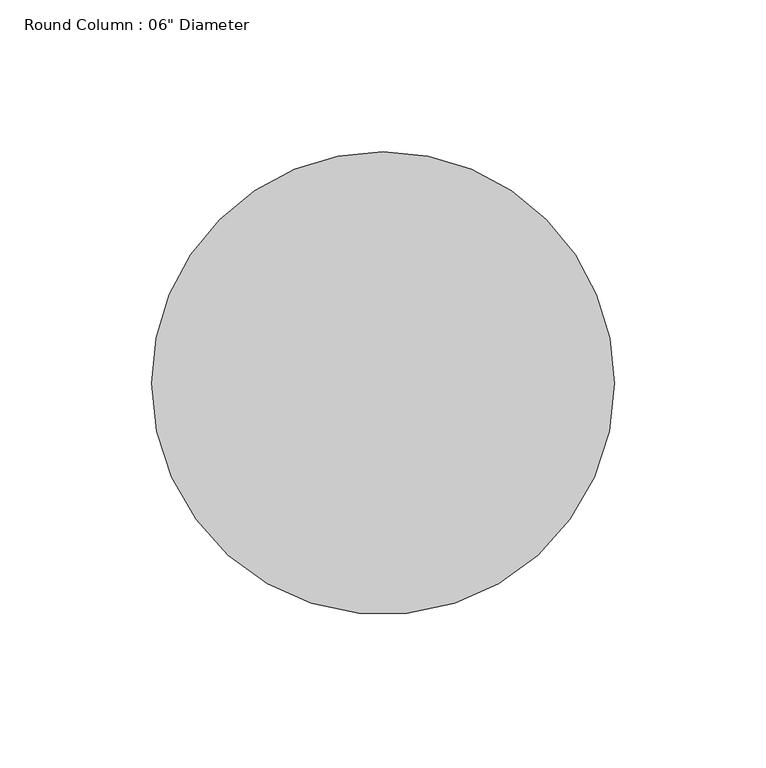
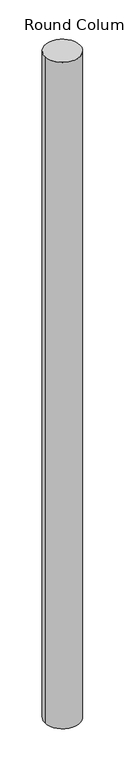
"""IFC4 building model written with IfcOpenShell, lengths in millimetres: column geometry."""

from ifc_helpers import new_model, si_unit, point, origin, origin_with_axes, origin_2d, place, context, project, spatial, circle_curve, trimmed, segment, composite_curve, outline, extrude, source, transform, mapped, element, save


def column_79e7fb11(model_context):
    return source(origin(), model_context, "Body", "SweptSolid", [
        extrude(outline(composite_curve([segment(trimmed(circle_curve(origin_2d(), 76.2), [point((76.2, 0.0))], [point((-76.2, 0.0))], False, "CARTESIAN"), True, "CONTINUOUS"), segment(trimmed(circle_curve(origin_2d(), 76.2), [point((-76.2, 0.0))], [point((0.0, 76.2))], False, "CARTESIAN"), True, "CONTINUOUS"), segment(trimmed(circle_curve(origin_2d(), 76.2), [point((0.0, 76.2))], [point((76.2, 0.0))], False, "CARTESIAN"), True, "CONTINUOUS")], self_intersect=False)), origin_with_axes(), (0.0, 0.0, 1.0), 3048.0),
    ])


if __name__ == "__main__":
    model = new_model("IFC4")
    model_context = context("Model", 3, world=origin())
    ifc_project = project(units=[si_unit("LENGTHUNIT", "METRE", prefix="MILLI")], contexts=[model_context])
    site = spatial("IfcSite", under=ifc_project)
    building = spatial("IfcBuilding", under=site)
    placement = place(None, origin())
    column_shape = column_79e7fb11(model_context)
    element("IfcColumn", 1, ObjectType="Round Column : 06\" Diameter", at=placement, inside=building, context=model_context, shape_type="MappedRepresentation", body=[
        mapped(column_shape, transform((0.0, 0.0, 0.0), x_axis=(1.0, 0.0, 0.0), y_axis=(0.0, 1.0, 0.0), z_axis=(0.0, 0.0, 1.0))),
    ])
    save(model, "model.ifc")

# Revit data of these elements
# Type "Round Column : 06\" Diameter"
#   Assembly Code = "B1010200"
#   Diameter = 0' - 6"
#   Offset Base = 0' - 0"
#   Offset Top = 0' - 0"
#   Material = none
